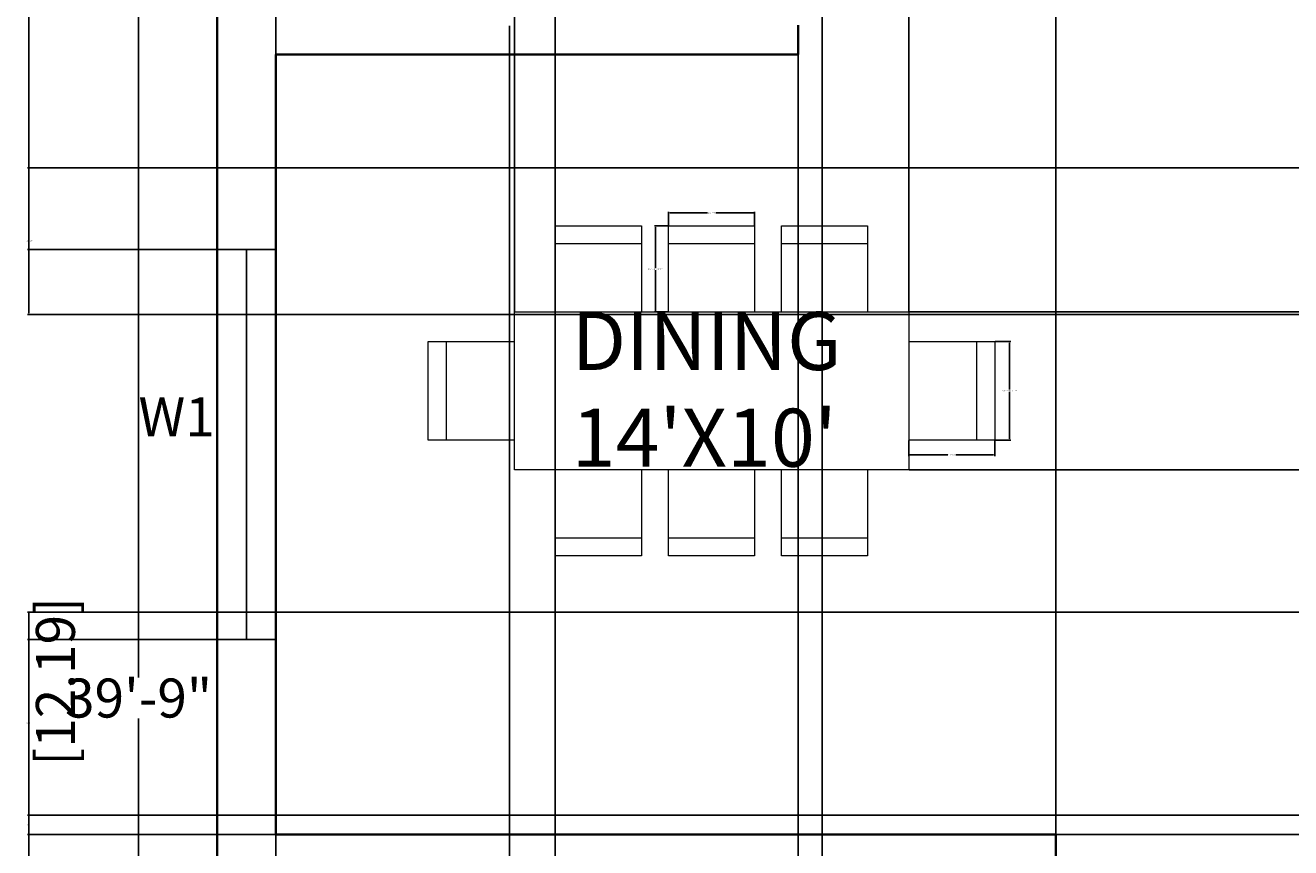
# Model space of a CAD drawing. Units: inches. Extents: x 3 to 420, y -502 to 54.
# Tile 4 of 6: x 3 to 198, y -257 to -130. Entities that reach past the tile are written whole.
import ezdxf

# ---------------------------------------------------------------- set-up
doc = ezdxf.new("R2010")
doc.units = ezdxf.units.IN
doc.header["$MEASUREMENT"] = 0
for name, color, linetype, lineweight in [('A-ANNO-DIMS', 2, 'Continuous', 18), ('A-ANNO-TEXT', 7, 'Continuous', 18), ('A-AREA-IDEN', 7, 'Continuous', 18), ('A-FURN', 8, 'Continuous', 18), ('A-GLAZ', 40, 'Continuous', 25), ('A-WALL', 7, 'Continuous', 35)]:
    doc.layers.add(name, color=color, linetype=linetype, lineweight=lineweight)
doc.styles.get("Standard").update_dxf_attribs({"font": 'arial.ttf'})
doc.dimstyles.get("Standard").update_dxf_attribs({"dimtxt": 0.18, "dimasz": 0.18, "dimexe": 0.18, "dimexo": 0.0625, "dimgap": 0.09, "dimtad": 0, "dimtih": 1, "dimtoh": 1, "dimdec": 0, "dimzin": 0, "dimdsep": 46, "dimlunit": 3, "dimtxsty": 'Standard', "dimcen": 0.09, "dimadec": 0, "dimazin": 0, "dimtfac": 1, "dimtdec": 0, "dimtofl": 0, "dimtmove": 0, "dimatfit": 3, "dimfxl": 1, "dimtolj": 1, "dimtzin": 0, "dimarcsym": 0})

# ---------------------------------------------------------------- blocks, each defined once
blk = doc.blocks.new('*D2')
at = {"layer": 'A-ANNO-DIMS', "color": 0, "lineweight": -2, "transparency": 16777216}
for p, q in [((32.33, 4.54), (20.1, 4.54)), ((20.28, 4.36), (20.28, -230.8)), ((20.28, -472.28), (20.28, -237.11)), ((32.33, -472.46), (20.1, -472.46))]:
    blk.add_line(p, q, dxfattribs=at)
at = {"layer": 'A-ANNO-DIMS', "color": 0, "transparency": 16777216}
for points in [[(20.25, 4.36), (20.31, 4.36), (20.28, 4.54)], [(20.25, -472.28), (20.31, -472.28), (20.28, -472.46)]]:
    blk.add_solid(points, dxfattribs=at)
at = {"layer": 'Defpoints', "color": 0, "transparency": 16777216}
for p in [(32.39, 4.54), (20.28, -472.46), (32.39, -472.46)]:
    blk.add_point(p, dxfattribs=at)
at = {"layer": 'A-ANNO-DIMS', "color": 0, "transparency": 16777216, "insert": (20.28, -233.96), "char_height": 6, "attachment_point": 5}
blk.add_mtext('\\A1;39\'-9"', dxfattribs=at)
blk = doc.blocks.new('WIN-W1-60')
for p, q in [((0, 9), (60, 9)), ((0, 9), (0, 0)), ((60, 9), (60, 0)), ((0, 4.5), (60, 4.5)), ((0, 0), (60, 0))]:
    blk.add_line(p, q)
blk = doc.blocks.new('CHAIR-DINING-SIDE')
for p, q in [((0, 0), (0, 13.24)), ((0, 13.24), (13.24, 13.24)), ((13.24, 13.24), (13.24, 0)), ((13.24, 10.48), (0, 10.48))]:
    blk.add_line(p, q)
blk = doc.blocks.new('CHAIR-DINING-END')
for p, q in [((0, 0), (0, 15.17)), ((0, 15.17), (13.24, 15.17)), ((2.76, 15.17), (2.76, 0)), ((13.24, 0), (0, 0))]:
    blk.add_line(p, q)
blk = doc.blocks.new('*D17')
at = {"layer": 'A-ANNO-DIMS', "color": 0, "lineweight": -2, "transparency": 16777216}
for p, q in [((101.75, -161.32), (99.64, -161.32)), ((99.82, -161.5), (99.82, -167.75)), ((99.82, -174.38), (99.82, -168.12)), ((101.75, -174.56), (99.64, -174.56))]:
    blk.add_line(p, q, dxfattribs=at)
at = {"layer": 'A-ANNO-DIMS', "color": 0, "transparency": 16777216}
for points in [[(99.79, -161.5), (99.85, -161.5), (99.82, -161.32)], [(99.79, -174.38), (99.85, -174.38), (99.82, -174.56)]]:
    blk.add_solid(points, dxfattribs=at)
at = {"layer": 'Defpoints', "color": 0, "transparency": 16777216}
for p in [(99.82, -161.32), (101.81, -161.32), (101.81, -174.56)]:
    blk.add_point(p, dxfattribs=at)
at = {"layer": 'A-ANNO-DIMS', "color": 0, "transparency": 16777216, "insert": (99.82, -167.94), "char_height": 0.18, "attachment_point": 5}
blk.add_mtext('\\A1;SIDE CHAIR 1\'-1" TYP.', dxfattribs=at)
blk = doc.blocks.new('*D18')
at = {"layer": 'A-ANNO-DIMS', "color": 0, "lineweight": -2, "transparency": 16777216}
for p, q in [((101.81, -161.25), (101.81, -159.15)), ((101.99, -159.33), (107.8, -159.33)), ((114.87, -159.33), (109.06, -159.33)), ((115.05, -161.25), (115.05, -159.15))]:
    blk.add_line(p, q, dxfattribs=at)
at = {"layer": 'A-ANNO-DIMS', "color": 0, "transparency": 16777216}
for points in [[(101.99, -159.3), (101.99, -159.36), (101.81, -159.33)], [(114.87, -159.3), (114.87, -159.36), (115.05, -159.33)]]:
    blk.add_solid(points, dxfattribs=at)
at = {"layer": 'Defpoints', "color": 0, "transparency": 16777216}
for p in [(115.05, -159.33), (101.81, -161.32), (115.05, -161.32)]:
    blk.add_point(p, dxfattribs=at)
at = {"layer": 'A-ANNO-DIMS', "color": 0, "transparency": 16777216, "insert": (108.43, -159.33), "char_height": 0.18, "attachment_point": 5}
blk.add_mtext('\\A1;1\'-1" TYP.', dxfattribs=at)
blk = doc.blocks.new('*D19')
at = {"layer": 'A-ANNO-DIMS', "color": 0, "lineweight": -2, "transparency": 16777216}
for p, q in [((152.07, -179.11), (154.46, -179.11)), ((154.28, -179.29), (154.28, -186.51)), ((154.28, -194.09), (154.28, -186.87)), ((152.07, -194.27), (154.46, -194.27))]:
    blk.add_line(p, q, dxfattribs=at)
at = {"layer": 'A-ANNO-DIMS', "color": 0, "transparency": 16777216}
for points in [[(154.25, -179.29), (154.31, -179.29), (154.28, -179.11)], [(154.25, -194.09), (154.31, -194.09), (154.28, -194.27)]]:
    blk.add_solid(points, dxfattribs=at)
at = {"layer": 'Defpoints', "color": 0, "transparency": 16777216}
for p in [(152, -179.11), (152, -194.27), (154.28, -194.27)]:
    blk.add_point(p, dxfattribs=at)
at = {"layer": 'A-ANNO-DIMS', "color": 0, "transparency": 16777216, "insert": (154.28, -186.69), "char_height": 0.18, "attachment_point": 5}
blk.add_mtext('\\A1;END CHAIR 1\'-3" TYP.', dxfattribs=at)
blk = doc.blocks.new('*D20')
at = {"layer": 'A-ANNO-DIMS', "color": 0, "lineweight": -2, "transparency": 16777216}
for p, q in [((138.77, -194.34), (138.77, -196.73)), ((152, -194.34), (152, -196.73)), ((138.95, -196.55), (144.75, -196.55)), ((151.82, -196.55), (146.01, -196.55))]:
    blk.add_line(p, q, dxfattribs=at)
at = {"layer": 'A-ANNO-DIMS', "color": 0, "transparency": 16777216}
for points in [[(138.95, -196.52), (138.95, -196.58), (138.77, -196.55)], [(151.82, -196.52), (151.82, -196.58), (152, -196.55)]]:
    blk.add_solid(points, dxfattribs=at)
at = {"layer": 'Defpoints', "color": 0, "transparency": 16777216}
for p in [(138.77, -194.27), (152, -194.27), (138.77, -196.55)]:
    blk.add_point(p, dxfattribs=at)
at = {"layer": 'A-ANNO-DIMS', "color": 0, "transparency": 16777216, "insert": (145.38, -196.55), "char_height": 0.18, "attachment_point": 5}
blk.add_mtext('\\A1;1\'-1" TYP.', dxfattribs=at)
blk = doc.blocks.new('*D39')
at = {"layer": 'A-ANNO-DIMS', "color": 0, "lineweight": -2, "transparency": 16777216}
for p, q in [((41.39, -130.52), (41.39, -501.64)), ((77.36, -130.52), (77.36, -501.64)), ((41.57, -501.46), (59.04, -501.46)), ((77.18, -501.46), (59.7, -501.46))]:
    blk.add_line(p, q, dxfattribs=at)
at = {"layer": 'A-ANNO-DIMS', "color": 0, "transparency": 16777216}
for points in [[(41.57, -501.43), (41.57, -501.49), (41.39, -501.46)], [(77.18, -501.43), (77.18, -501.49), (77.36, -501.46)]]:
    blk.add_solid(points, dxfattribs=at)
at = {"layer": 'Defpoints', "color": 0, "transparency": 16777216}
for p in [(41.39, -130.46), (77.36, -130.46), (77.36, -501.46)]:
    blk.add_point(p, dxfattribs=at)
at = {"layer": 'A-ANNO-DIMS', "color": 0, "transparency": 16777216, "insert": (59.37, -501.46), "char_height": 0.18, "attachment_point": 5}
blk.add_mtext('\\A1;3\'-0"', dxfattribs=at)
blk = doc.blocks.new('*D45')
at = {"layer": 'A-ANNO-DIMS', "color": 0, "lineweight": -2, "transparency": 16777216}
for p, q in [((41.39, -130.39), (41.39, 33.72)), ((41.57, 33.54), (42.12, 33.54)), ((43.75, 33.54), (43.2, 33.54)), ((43.93, -109.33), (43.93, 33.72))]:
    blk.add_line(p, q, dxfattribs=at)
at = {"layer": 'A-ANNO-DIMS', "color": 0, "transparency": 16777216}
for points in [[(41.57, 33.57), (41.57, 33.51), (41.39, 33.54)], [(43.75, 33.57), (43.75, 33.51), (43.93, 33.54)]]:
    blk.add_solid(points, dxfattribs=at)
at = {"layer": 'Defpoints', "color": 0, "transparency": 16777216}
for p in [(41.39, 33.54), (43.93, -109.39), (41.39, -130.46)]:
    blk.add_point(p, dxfattribs=at)
at = {"layer": 'A-ANNO-DIMS', "color": 0, "transparency": 16777216, "insert": (42.66, 33.54), "char_height": 0.18, "attachment_point": 5}
blk.add_mtext('\\A1;0\'-2 1/2"', dxfattribs=at)
blk = doc.blocks.new('*D46')
at = {"layer": 'A-ANNO-DIMS', "color": 0, "lineweight": -2, "transparency": 16777216}
for p, q in [((41.39, -135.02), (41.39, -501.64)), ((121.75, -135.02), (121.75, -501.64)), ((41.57, -501.46), (81.03, -501.46)), ((121.57, -501.46), (82.11, -501.46))]:
    blk.add_line(p, q, dxfattribs=at)
at = {"layer": 'A-ANNO-DIMS', "color": 0, "transparency": 16777216}
for points in [[(41.57, -501.43), (41.57, -501.49), (41.39, -501.46)], [(121.57, -501.43), (121.57, -501.49), (121.75, -501.46)]]:
    blk.add_solid(points, dxfattribs=at)
at = {"layer": 'Defpoints', "color": 0, "transparency": 16777216}
for p in [(41.39, -134.96), (121.75, -134.96), (121.75, -501.46)]:
    blk.add_point(p, dxfattribs=at)
at = {"layer": 'A-ANNO-DIMS', "color": 0, "transparency": 16777216, "insert": (81.57, -501.46), "char_height": 0.18, "attachment_point": 5}
blk.add_mtext('\\A1;6\'-8 1/2"', dxfattribs=at)
blk = doc.blocks.new('*D47')
at = {"layer": 'A-ANNO-DIMS', "color": 0, "lineweight": -2, "transparency": 16777216}
for p, q in [((41.39, -254.89), (41.39, 33.72)), ((41.57, 33.54), (101, 33.54)), ((161.2, 33.54), (101.78, 33.54)), ((161.38, -254.89), (161.38, 33.72))]:
    blk.add_line(p, q, dxfattribs=at)
at = {"layer": 'A-ANNO-DIMS', "color": 0, "transparency": 16777216}
for points in [[(41.57, 33.57), (41.57, 33.51), (41.39, 33.54)], [(161.2, 33.57), (161.2, 33.51), (161.38, 33.54)]]:
    blk.add_solid(points, dxfattribs=at)
at = {"layer": 'Defpoints', "color": 0, "transparency": 16777216}
for p in [(161.38, 33.54), (41.39, -254.96), (161.38, -254.96)]:
    blk.add_point(p, dxfattribs=at)
at = {"layer": 'A-ANNO-DIMS', "color": 0, "transparency": 16777216, "insert": (101.39, 33.54), "char_height": 0.18, "attachment_point": 5}
blk.add_mtext('\\A1;10\'-0"', dxfattribs=at)
blk = doc.blocks.new('*D60')
at = {"layer": 'A-ANNO-DIMS', "color": 0, "lineweight": -2, "transparency": 16777216}
for p, q in [((32.33, -85.46), (3.21, -85.46)), ((3.39, -85.64), (3.39, -125.02)), ((3.39, -164.78), (3.39, -125.39)), ((32.33, -164.96), (3.21, -164.96))]:
    blk.add_line(p, q, dxfattribs=at)
at = {"layer": 'A-ANNO-DIMS', "color": 0, "transparency": 16777216}
for points in [[(3.36, -85.64), (3.42, -85.64), (3.39, -85.46)], [(3.36, -164.78), (3.42, -164.78), (3.39, -164.96)]]:
    blk.add_solid(points, dxfattribs=at)
at = {"layer": 'Defpoints', "color": 0, "transparency": 16777216}
for p in [(32.39, -85.46), (3.39, -164.96), (32.39, -164.96)]:
    blk.add_point(p, dxfattribs=at)
at = {"layer": 'A-ANNO-DIMS', "color": 0, "transparency": 16777216, "insert": (3.39, -125.21), "char_height": 0.18, "attachment_point": 5}
blk.add_mtext('\\A1;6\'-7 1/2"', dxfattribs=at)
blk = doc.blocks.new('*D61')
at = {"layer": 'A-ANNO-DIMS', "color": 0, "lineweight": -2, "transparency": 16777216}
for p, q in [((32.33, -224.96), (3.21, -224.96)), ((3.39, -225.14), (3.39, -280.27)), ((3.39, -335.78), (3.39, -280.64)), ((32.33, -335.96), (3.21, -335.96))]:
    blk.add_line(p, q, dxfattribs=at)
at = {"layer": 'A-ANNO-DIMS', "color": 0, "transparency": 16777216}
for points in [[(3.36, -225.14), (3.42, -225.14), (3.39, -224.96)], [(3.36, -335.78), (3.42, -335.78), (3.39, -335.96)]]:
    blk.add_solid(points, dxfattribs=at)
at = {"layer": 'Defpoints', "color": 0, "transparency": 16777216}
for p in [(32.39, -224.96), (3.39, -335.96), (32.39, -335.96)]:
    blk.add_point(p, dxfattribs=at)
at = {"layer": 'A-ANNO-DIMS', "color": 0, "transparency": 16777216, "insert": (3.39, -280.46), "char_height": 0.18, "attachment_point": 5}
blk.add_mtext('\\A1;9\'-3"', dxfattribs=at)
blk = doc.blocks.new('*D62')
at = {"layer": 'A-ANNO-DIMS', "color": 0, "lineweight": -2, "transparency": 16777216}
for p, q in [((84.39, -463.39), (84.39, 33.72)), ((84.57, 33.54), (104.58, 33.54)), ((125.25, 33.54), (105.24, 33.54)), ((125.43, -463.39), (125.43, 33.72))]:
    blk.add_line(p, q, dxfattribs=at)
at = {"layer": 'A-ANNO-DIMS', "color": 0, "transparency": 16777216}
for points in [[(84.57, 33.57), (84.57, 33.51), (84.39, 33.54)], [(125.25, 33.57), (125.25, 33.51), (125.43, 33.54)]]:
    blk.add_solid(points, dxfattribs=at)
at = {"layer": 'Defpoints', "color": 0, "transparency": 16777216}
for p in [(125.43, 33.54), (84.39, -463.46), (125.43, -463.46)]:
    blk.add_point(p, dxfattribs=at)
at = {"layer": 'A-ANNO-DIMS', "color": 0, "transparency": 16777216, "insert": (104.91, 33.54), "char_height": 0.18, "attachment_point": 5}
blk.add_mtext('\\A1;3\'-5"', dxfattribs=at)
blk = doc.blocks.new('*D70')
at = {"layer": 'A-ANNO-DIMS', "color": 0, "lineweight": -2, "transparency": 16777216}
for p, q in [((310.7, -152.37), (3.21, -152.37)), ((3.39, -152.55), (3.39, -163.47)), ((3.39, -174.75), (3.39, -163.83)), ((310.9, -174.93), (3.21, -174.93))]:
    blk.add_line(p, q, dxfattribs=at)
at = {"layer": 'A-ANNO-DIMS', "color": 0, "transparency": 16777216}
for points in [[(3.36, -152.55), (3.42, -152.55), (3.39, -152.37)], [(3.36, -174.75), (3.42, -174.75), (3.39, -174.93)]]:
    blk.add_solid(points, dxfattribs=at)
at = {"layer": 'Defpoints', "color": 0, "transparency": 16777216}
for p in [(3.39, -152.37), (310.77, -152.37), (310.96, -174.93)]:
    blk.add_point(p, dxfattribs=at)
at = {"layer": 'A-ANNO-DIMS', "color": 0, "transparency": 16777216, "insert": (3.39, -163.65), "char_height": 0.18, "attachment_point": 5}
blk.add_mtext('\\A1;1\'-10 1/2"', dxfattribs=at)
blk = doc.blocks.new('*D71')
at = {"layer": 'A-ANNO-DIMS', "color": 0, "lineweight": -2, "transparency": 16777216}
for p, q in [((78.09, -174.49), (78.09, 33.72)), ((78.27, 33.54), (107.89, 33.54)), ((138.59, 33.54), (108.97, 33.54)), ((138.77, -174.49), (138.77, 33.72))]:
    blk.add_line(p, q, dxfattribs=at)
at = {"layer": 'A-ANNO-DIMS', "color": 0, "transparency": 16777216}
for points in [[(78.27, 33.57), (78.27, 33.51), (78.09, 33.54)], [(138.59, 33.57), (138.59, 33.51), (138.77, 33.54)]]:
    blk.add_solid(points, dxfattribs=at)
at = {"layer": 'Defpoints', "color": 0, "transparency": 16777216}
for p in [(138.77, 33.54), (78.09, -174.56), (138.77, -174.56)]:
    blk.add_point(p, dxfattribs=at)
at = {"layer": 'A-ANNO-DIMS', "color": 0, "transparency": 16777216, "insert": (108.43, 33.54), "char_height": 0.18, "attachment_point": 5}
blk.add_mtext('\\A1;5\'-0 1/2"', dxfattribs=at)
blk = doc.blocks.new('*D72')
at = {"layer": 'A-ANNO-DIMS', "color": 0, "lineweight": -2, "transparency": 16777216}
for p, q in [((138.83, -174.56), (420.07, -174.56)), ((419.89, -174.74), (419.89, -186.51)), ((419.89, -198.65), (419.89, -186.87)), ((138.83, -198.83), (420.07, -198.83))]:
    blk.add_line(p, q, dxfattribs=at)
at = {"layer": 'A-ANNO-DIMS', "color": 0, "transparency": 16777216}
for points in [[(419.86, -174.74), (419.92, -174.74), (419.89, -174.56)], [(419.86, -198.65), (419.92, -198.65), (419.89, -198.83)]]:
    blk.add_solid(points, dxfattribs=at)
at = {"layer": 'Defpoints', "color": 0, "transparency": 16777216}
for p in [(138.77, -174.56), (138.77, -198.83), (419.89, -198.83)]:
    blk.add_point(p, dxfattribs=at)
at = {"layer": 'A-ANNO-DIMS', "color": 0, "transparency": 16777216, "insert": (419.89, -186.69), "char_height": 0.18, "attachment_point": 5}
blk.add_mtext('\\A1;2\'-0 1/2"', dxfattribs=at)
blk = doc.blocks.new('*D76')
at = {"layer": 'A-ANNO-DIMS', "color": 0, "lineweight": -2, "transparency": 16777216}
for p, q in [((358.46, -220.72), (3.21, -220.72)), ((3.39, -220.9), (3.39, -237.66)), ((3.39, -254.78), (3.39, -238.02)), ((365, -254.96), (3.21, -254.96))]:
    blk.add_line(p, q, dxfattribs=at)
at = {"layer": 'A-ANNO-DIMS', "color": 0, "transparency": 16777216}
for points in [[(3.36, -220.9), (3.42, -220.9), (3.39, -220.72)], [(3.36, -254.78), (3.42, -254.78), (3.39, -254.96)]]:
    blk.add_solid(points, dxfattribs=at)
at = {"layer": 'Defpoints', "color": 0, "transparency": 16777216}
for p in [(358.53, -220.72), (3.39, -254.96), (365.06, -254.96)]:
    blk.add_point(p, dxfattribs=at)
at = {"layer": 'A-ANNO-DIMS', "color": 0, "transparency": 16777216, "insert": (3.39, -237.84), "char_height": 0.18, "attachment_point": 5}
blk.add_mtext('\\A1;2\'-10"', dxfattribs=at)
blk = doc.blocks.new('*D81')
at = {"layer": 'A-ANNO-DIMS', "color": 0, "lineweight": -2, "transparency": 16777216}
for p, q in [((309.83, -251.96), (3.21, -251.96)), ((3.39, -252.14), (3.39, -253.27)), ((309.83, -254.96), (3.21, -254.96)), ((3.39, -254.78), (3.39, -253.64))]:
    blk.add_line(p, q, dxfattribs=at)
at = {"layer": 'A-ANNO-DIMS', "color": 0, "transparency": 16777216}
for points in [[(3.36, -252.14), (3.42, -252.14), (3.39, -251.96)], [(3.36, -254.78), (3.42, -254.78), (3.39, -254.96)]]:
    blk.add_solid(points, dxfattribs=at)
at = {"layer": 'Defpoints', "color": 0, "transparency": 16777216}
for p in [(309.89, -251.96), (3.39, -254.96), (309.89, -254.96)]:
    blk.add_point(p, dxfattribs=at)
at = {"layer": 'A-ANNO-DIMS', "color": 0, "transparency": 16777216, "insert": (3.39, -253.46), "char_height": 0.18, "attachment_point": 5}
blk.add_mtext('\\A1;0\'-3"', dxfattribs=at)

msp = doc.modelspace()

# ---------------------------------------------------------------- linework, layer by layer
at = {"layer": 'A-FURN'}
for p, q in [((78.09, -174.56), (138.77, -174.56)), ((78.09, -198.83), (78.09, -174.56)), ((138.77, -174.56), (138.77, -198.83)), ((138.77, -198.83), (78.09, -198.83))]:
    msp.add_line(p, q, dxfattribs=at)
at = {"layer": 'A-WALL'}
for p, q in [((32.39, 4.54), (32.39, -472.46)), ((121.75, -130.46), (121.75, -134.96)), ((41.39, -134.96), (121.75, -134.96)), ((41.39, -134.96), (41.39, -254.96)), ((41.39, -254.96), (161.38, -254.96)), ((161.38, -254.96), (161.38, -259.46))]:
    msp.add_line(p, q, dxfattribs=at)

# ---------------------------------------------------------------- block references
at = {"layer": 'A-FURN'}
for name, p in [('CHAIR-DINING-SIDE', (84.43, -174.56)), ('CHAIR-DINING-SIDE', (101.81, -174.56)), ('CHAIR-DINING-SIDE', (119.18, -174.56)), ('CHAIR-DINING-END', (64.85, -194.28))]:
    msp.add_blockref(name, p, dxfattribs=at)
at = {"layer": 'A-FURN', "rotation": 180}
for name, p in [('CHAIR-DINING-END', (152, -179.11)), ('CHAIR-DINING-SIDE', (97.67, -198.83)), ('CHAIR-DINING-SIDE', (115.05, -198.83)), ('CHAIR-DINING-SIDE', (132.42, -198.83))]:
    msp.add_blockref(name, p, dxfattribs=at)
at = {"layer": 'A-GLAZ', "rotation": 269.9999999999999}
msp.add_blockref('WIN-W1-60', (32.39, -164.96), dxfattribs=at)

# ---------------------------------------------------------------- texts
at = {"layer": 'A-ANNO-DIMS', "insert": (4.49, -244.38), "char_height": 6, "attachment_point": 1, "rotation": 90}
msp.add_mtext('[12.19]', dxfattribs=at)
at = {"layer": 'A-ANNO-TEXT', "insert": (20.27, -187.69), "char_height": 6, "attachment_point": 1}
msp.add_mtext('W1', dxfattribs=at)
at = {"layer": 'A-AREA-IDEN', "insert": (86.91, -174.56), "char_height": 8.929, "attachment_point": 1}
msp.add_mtext("DINING\\P14'X10'", dxfattribs=at)

# ---------------------------------------------------------------- dimensions: what is measured, and where the dimension line sits
at = {"layer": 'A-ANNO-DIMS'}
for base, p1, p2, picture, middle in [((41.39, 33.54), (43.93, -109.39), (41.39, -130.46), '*D45', (42.66, 33.54)), ((161.38, 33.54), (41.39, -254.96), (161.38, -254.96), '*D47', (101.39, 33.54)), ((138.77, 33.54), (78.09, -174.56), (138.77, -174.56), '*D71', (108.43, 33.54)), ((125.43, 33.54), (84.39, -463.46), (125.43, -463.46), '*D62', (104.91, 33.54)), ((77.36, -501.46), (41.39, -130.46), (77.36, -130.46), '*D39', (59.37, -501.46)), ((121.75, -501.46), (41.39, -134.96), (121.75, -134.96), '*D46', (81.57, -501.46))]:
    dim = msp.add_linear_dim(base=base, p1=p1, p2=p2, dimstyle='Standard', override={"dimdec": 1, "dimlfac": 1, "dimrnd": 0, "dimzin": 1, "dimdsep": 46, "dimlunit": 4, "dimfrac": 2}, dxfattribs=at)
    dim.commit()
    dim.dimension.update_dxf_attribs({"geometry": picture, "text_midpoint": middle})
for base, p1, p2, override, picture, middle in [((20.28, -472.46), (32.39, 4.54), (32.39, -472.46), {"dimtxt": 6, "dimclrd": 0, "dimclre": 0, "dimclrt": 0}, '*D2', (20.28, -233.96)), ((3.39, -164.96), (32.39, -85.46), (32.39, -164.96), {"dimdec": 1, "dimlfac": 1, "dimrnd": 0, "dimzin": 1, "dimdsep": 46, "dimlunit": 4, "dimfrac": 2}, '*D60', (3.39, -125.21)), ((3.39, -152.37), (310.96, -174.93), (310.77, -152.37), {"dimdec": 1, "dimlfac": 1, "dimrnd": 0, "dimzin": 1, "dimdsep": 46, "dimlunit": 4, "dimfrac": 2}, '*D70', (3.39, -163.65)), ((419.89, -198.83), (138.77, -174.56), (138.77, -198.83), {"dimdec": 1, "dimlfac": 1, "dimrnd": 0, "dimzin": 1, "dimdsep": 46, "dimlunit": 4, "dimfrac": 2}, '*D72', (419.89, -186.69)), ((3.39, -254.96), (358.53, -220.72), (365.06, -254.96), {"dimdec": 1, "dimlfac": 1, "dimrnd": 0, "dimzin": 1, "dimdsep": 46, "dimlunit": 4, "dimfrac": 2}, '*D76', (3.39, -237.84)), ((3.39, -335.96), (32.39, -224.96), (32.39, -335.96), {"dimdec": 1, "dimlfac": 1, "dimrnd": 0, "dimzin": 1, "dimdsep": 46, "dimlunit": 4, "dimfrac": 2}, '*D61', (3.39, -280.46)), ((3.39, -254.96), (309.89, -251.96), (309.89, -254.96), {"dimdec": 1, "dimlfac": 1, "dimrnd": 0, "dimzin": 1, "dimdsep": 46, "dimlunit": 4, "dimfrac": 2}, '*D81', (3.39, -253.46))]:
    dim = msp.add_linear_dim(base=base, p1=p1, p2=p2, angle=90, dimstyle='Standard', override=override, dxfattribs=at)
    dim.commit()
    dim.dimension.update_dxf_attribs({"geometry": picture, "text_midpoint": middle})
dim = msp.add_linear_dim(base=(115.05, -159.33), p1=(101.81, -161.32), p2=(115.05, -161.32), text='<> TYP.', dimstyle='Standard', override={"dimdec": 1, "dimlfac": 1, "dimrnd": 0, "dimzin": 1, "dimdsep": 46, "dimlunit": 4, "dimfrac": 2}, dxfattribs=at)
dim.commit()
dim.dimension.update_dxf_attribs({"geometry": '*D18', "text_midpoint": (108.43, -159.33)})
for base, p1, p2, angle, text, picture, middle in [((99.82, -161.32), (101.81, -174.56), (101.81, -161.32), 90, 'SIDE CHAIR <> TYP.', '*D17', (99.82, -167.94)), ((154.28, -194.27), (152, -179.11), (152, -194.27), 270, 'END CHAIR <> TYP.', '*D19', (154.28, -186.69)), ((138.77, -196.55), (152, -194.27), (138.77, -194.27), 180, '<> TYP.', '*D20', (145.38, -196.55))]:
    dim = msp.add_linear_dim(base=base, p1=p1, p2=p2, angle=angle, text=text, dimstyle='Standard', override={"dimdec": 1, "dimlfac": 1, "dimrnd": 0, "dimzin": 1, "dimdsep": 46, "dimlunit": 4, "dimfrac": 2}, dxfattribs=at)
    dim.commit()
    dim.dimension.update_dxf_attribs({"geometry": picture, "text_midpoint": middle})

doc.saveas('drawing.dxf')
